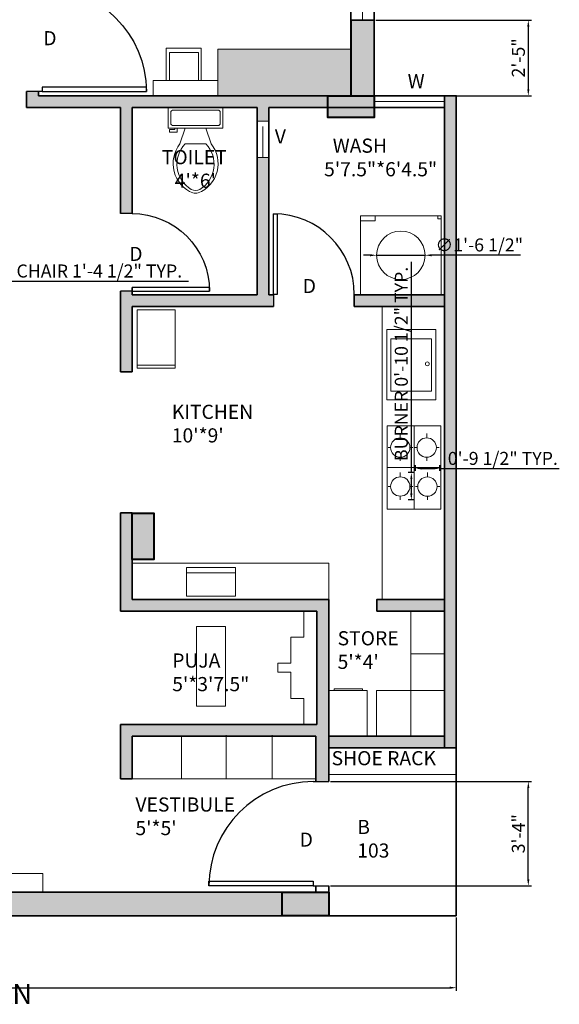
# Model space of a CAD drawing. Units: inches. Extents: x 351 to 1945, y 4338 to 4989.
# Tile 2 of 4: x 633 to 841, y 4338 to 4716. Entities that reach past the tile are written whole.
import ezdxf

# ---------------------------------------------------------------- set-up
doc = ezdxf.new("R2010")
doc.units = ezdxf.units.IN
doc.linetypes.add('ACAD_ISO02W100', pattern=[15, 12, -3])
for name, color, linetype, lineweight in [('A-ANNO-DIMS', 55, 'Continuous', 18), ('A-ANNO-IDEN', 55, 'Continuous', 18), ('A-ANNO-TEXT', 55, 'Continuous', 25), ('A-AREA-IDEN', 55, 'Continuous', 18), ('A-COLS-PATT', 210, 'Continuous', 13), ('A-EQPM', 8, 'Continuous', 18), ('A-FLOR-CASE', 30, 'Continuous', 20), ('A-FLOR-CASE-PATT', 30, 'Continuous', 13), ('A-FLOR-FIXT', 9, 'Continuous', 18), ('A-GLAZ-HIDN', 10, 'ACAD_ISO02W100', 18), ('A-WALL-PATT', 130, 'Continuous', 13), ('COLUMN', 210, 'Continuous', 40), ('DOOR', 52, 'Continuous', 25), ('FUR', 142, 'Continuous', 18), ('WALL', 130, 'Continuous', 35), ('WIND', 10, 'Continuous', 20)]:
    doc.layers.add(name, color=color, linetype=linetype, lineweight=lineweight)
doc.styles.get("Standard").update_dxf_attribs({"font": 'arial.ttf'})
doc.dimstyles.new('ISO-25', dxfattribs={"dimtxt": 5, "dimasz": 2.5, "dimexe": 1.25, "dimexo": 0.625, "dimtad": 1, "dimdec": 0, "dimlunit": 4, "dimtxsty": 'Standard', "dimcen": 2.5, "dimadec": 0, "dimazin": 0, "dimtfac": 1, "dimtdec": 0, "dimtmove": 0, "dimatfit": 3, "dimfxl": 1, "dimarcsym": 0})

# ---------------------------------------------------------------- blocks, each defined once
blk = doc.blocks.new('*U2')
for p, q in [((0, 0), (0, -6)), ((40, 0), (40, -6))]:
    blk.add_line(p, q)
blk.add_lwpolyline([(0, 0), (0, 40), (1.75, 40), (1.75, 0)], close=True)
blk.add_arc((0, 0), 40, 0, 90)
blk = doc.blocks.new('*U4')
for p, q in [((9.5, -6), (9.5, -2)), ((-10, -8.5), (-8, -8.5)), ((-10, -9.5), (-10, -8.5)), ((-7, -9.5), (-10, -9.5)), ((-8, -8.5), (-8, -8)), ((-7, -8), (-7, -9.5)), ((-4, -8), (-6, -14)), ((4, -8), (6, -14)), ((4, -14), (-4, -14))]:
    blk.add_line(p, q)
blk.add_lwpolyline([(10.5, -8), (10.5, 0), (-10.5, 0), (-10.5, -8)], close=True)
for points in [[(-9.5, -2), (-9.5, -6)], [(8.5, -1), (-8.5, -1)], [(-8.5, -7), (8.5, -7)]]:
    blk.add_lwpolyline(points)
for centre, radius, start, end in [((-8.62, -1.88), 0.884, 81.8699, 188.1301), ((8.62, -1.88), 0.884, 351.8699, 98.1301), ((-8.62, -6.12), 0.884, 171.8699, 278.1301), ((8.62, -6.12), 0.884, 261.8699, 8.1301), ((3.52, -21.58), 12.17, 141.4691, 247.9714), ((4.2, -21.82), 11.33, 136.3677, 238.9468), ((-3.52, -21.58), 12.17, 292.0284, 38.5307), ((-4.2, -21.82), 11.33, 301.053, 43.6321), ((0, -27.88), 4, 245.7318, 294.2682), ((0, -29), 4, 254.8605, 285.1395)]:
    blk.add_arc(centre, radius, start, end)
blk = doc.blocks.new('BEDROOM-DESK-AND-SEAT')
for p, q in [((5, 5.84), (5, 18.2)), ((5, 18.2), (18.5, 18.2)), ((18.5, 18.2), (18.5, 5.84))]:
    blk.add_line(p, q)
for points in [[(6.28, 5.84), (17.4, 5.84), (17.4, 16.62), (6.28, 16.62)], [(0, 0), (24.89, 0), (24.89, 5.84), (0, 5.84)]]:
    blk.add_lwpolyline(points, close=True)
blk = doc.blocks.new('WIN-49')
blk.add_line((0, 4.5), (49.03, 4.5))
blk.add_lwpolyline([(0, 0), (49.03, 0), (49.03, 9), (0, 9)], close=True)
blk = doc.blocks.new('COOKTOP-BURNER')
for p, q in [((4.6, 8.82), (4.6, 10.51)), ((0.89, 5.11), (0, 5.11)), ((8.32, 5.11), (9.37, 5.11)), ((4.6, 1.39), (4.6, 0))]:
    blk.add_line(p, q)
blk.add_circle((4.6, 5.11), 3.72)
blk = doc.blocks.new('*D15')
at = {"layer": 'A-ANNO-DIMS', "color": 0, "lineweight": -2, "transparency": 16777216}
for p, q in [((586.22, 4617.77), (586.22, 4614.71)), ((588.72, 4615.96), (599.99, 4615.96)), ((602.49, 4617.77), (602.49, 4614.71)), ((602.49, 4615.96), (698.18, 4615.96))]:
    blk.add_line(p, q, dxfattribs=at)
at = {"layer": 'A-ANNO-DIMS', "color": 0, "lineweight": 100, "transparency": 16777216}
for points in [[(588.72, 4616.38), (588.72, 4615.54), (586.22, 4615.96)], [(599.99, 4616.38), (599.99, 4615.54), (602.49, 4615.96)]]:
    blk.add_solid(points, dxfattribs=at)
at = {"layer": 'Defpoints', "color": 0, "lineweight": 100, "transparency": 16777216}
for p in [(586.22, 4618.4), (602.49, 4618.4), (602.49, 4615.96)]:
    blk.add_point(p, dxfattribs=at)
at = {"layer": 'A-ANNO-DIMS', "color": 0, "transparency": 16777216, "insert": (651.59, 4619.17), "char_height": 5, "attachment_point": 5}
blk.add_mtext('DINING CHAIR 1\'-4 1/2" TYP.', dxfattribs=at)
blk = doc.blocks.new('*D19')
at = {"layer": 'A-ANNO-DIMS', "color": 0, "lineweight": -2, "transparency": 16777216}
for p, q in [((783.81, 4542.4), (783.81, 4623.38)), ((784.76, 4542.4), (782.56, 4542.4)), ((783.81, 4534.39), (783.81, 4539.9)), ((784.76, 4531.89), (782.56, 4531.89))]:
    blk.add_line(p, q, dxfattribs=at)
at = {"layer": 'A-ANNO-DIMS', "color": 0, "lineweight": 100, "transparency": 16777216}
for points in [[(783.39, 4539.9), (784.22, 4539.9), (783.81, 4542.4)], [(783.39, 4534.39), (784.22, 4534.39), (783.81, 4531.89)]]:
    blk.add_solid(points, dxfattribs=at)
at = {"layer": 'Defpoints', "color": 0, "lineweight": 100, "transparency": 16777216}
for p in [(783.81, 4542.4), (785.38, 4542.4), (785.38, 4531.89)]:
    blk.add_point(p, dxfattribs=at)
at = {"layer": 'A-ANNO-DIMS', "color": 0, "transparency": 16777216, "insert": (780.6, 4584.14), "char_height": 5, "attachment_point": 5, "rotation": 90}
blk.add_mtext('BURNER 0\'-10 1/2" TYP.', dxfattribs=at)
blk = doc.blocks.new('*D20')
at = {"layer": 'A-ANNO-DIMS', "color": 0, "lineweight": -2, "transparency": 16777216}
for p, q in [((785.38, 4543.02), (785.38, 4545.23)), ((787.88, 4543.98), (792.26, 4543.98)), ((794.76, 4543.02), (794.76, 4545.23)), ((794.76, 4543.98), (840.64, 4543.98))]:
    blk.add_line(p, q, dxfattribs=at)
at = {"layer": 'A-ANNO-DIMS', "color": 0, "lineweight": 100, "transparency": 16777216}
for points in [[(787.88, 4544.39), (787.88, 4543.56), (785.38, 4543.98)], [(792.26, 4544.39), (792.26, 4543.56), (794.76, 4543.98)]]:
    blk.add_solid(points, dxfattribs=at)
at = {"layer": 'Defpoints', "color": 0, "lineweight": 100, "transparency": 16777216}
for p in [(794.76, 4543.98), (785.38, 4542.4), (794.76, 4542.4)]:
    blk.add_point(p, dxfattribs=at)
at = {"layer": 'A-ANNO-DIMS', "color": 0, "transparency": 16777216, "insert": (818.95, 4547.19), "char_height": 5, "attachment_point": 5}
blk.add_mtext('0\'-9 1/2" TYP.', dxfattribs=at)
blk = doc.blocks.new('*D31')
at = {"layer": 'A-ANNO-DIMS', "color": 0, "lineweight": -2, "transparency": 16777216}
for p, q in [((402.08, 4469.03), (402.08, 4343.26)), ((801.08, 4371.53), (801.08, 4343.26)), ((404.58, 4344.51), (798.58, 4344.51))]:
    blk.add_line(p, q, dxfattribs=at)
at = {"layer": 'A-ANNO-DIMS', "color": 0, "lineweight": 100, "transparency": 16777216}
for points in [[(404.58, 4344.93), (404.58, 4344.09), (402.08, 4344.51)], [(798.58, 4344.93), (798.58, 4344.09), (801.08, 4344.51)]]:
    blk.add_solid(points, dxfattribs=at)
at = {"layer": 'Defpoints', "color": 0, "lineweight": 100, "transparency": 16777216}
for p in [(402.08, 4469.66), (801.08, 4372.16), (801.08, 4344.51)]:
    blk.add_point(p, dxfattribs=at)
at = {"layer": 'A-ANNO-DIMS', "color": 0, "transparency": 16777216, "insert": (601.58, 4347.69), "char_height": 5, "attachment_point": 5}
blk.add_mtext('33\'-3"', dxfattribs=at)
blk = doc.blocks.new('*D32')
at = {"layer": 'A-ANNO-DIMS', "color": 0, "lineweight": -2, "transparency": 16777216}
for p, q in [((770.21, 4716.2), (829.98, 4716.2)), ((828.73, 4713.7), (828.73, 4689.66)), ((770.21, 4687.16), (829.98, 4687.16))]:
    blk.add_line(p, q, dxfattribs=at)
at = {"layer": 'A-ANNO-DIMS', "color": 0, "lineweight": 100, "transparency": 16777216}
for points in [[(828.32, 4713.7), (829.15, 4713.7), (828.73, 4716.2)], [(828.32, 4689.66), (829.15, 4689.66), (828.73, 4687.16)]]:
    blk.add_solid(points, dxfattribs=at)
at = {"layer": 'Defpoints', "color": 0, "lineweight": 100, "transparency": 16777216}
for p in [(769.58, 4716.2), (769.58, 4687.16), (828.73, 4687.16)]:
    blk.add_point(p, dxfattribs=at)
at = {"layer": 'A-ANNO-DIMS', "color": 0, "transparency": 16777216, "insert": (825.56, 4701.68), "char_height": 5, "attachment_point": 5, "rotation": 90}
blk.add_mtext('2\'-5"', dxfattribs=at)
blk = doc.blocks.new('*D38')
at = {"layer": 'A-ANNO-DIMS', "color": 0, "lineweight": -2, "transparency": 16777216}
for p, q in [((752.71, 4423.66), (829.98, 4423.66)), ((828.73, 4386.16), (828.73, 4421.16)), ((752.71, 4383.66), (829.98, 4383.66))]:
    blk.add_line(p, q, dxfattribs=at)
at = {"layer": 'A-ANNO-DIMS', "color": 0, "lineweight": 100, "transparency": 16777216}
for points in [[(828.32, 4421.16), (829.15, 4421.16), (828.73, 4423.66)], [(828.32, 4386.16), (829.15, 4386.16), (828.73, 4383.66)]]:
    blk.add_solid(points, dxfattribs=at)
at = {"layer": 'Defpoints', "color": 0, "lineweight": 100, "transparency": 16777216}
for p in [(752.08, 4423.66), (828.73, 4423.66), (752.08, 4383.66)]:
    blk.add_point(p, dxfattribs=at)
at = {"layer": 'A-ANNO-DIMS', "color": 0, "transparency": 16777216, "insert": (825.56, 4403.66), "char_height": 5, "attachment_point": 5, "rotation": 90}
blk.add_mtext('3\'-4"', dxfattribs=at)
blk = doc.blocks.new('*D52')
at = {"layer": 'A-ANNO-DIMS', "color": 0, "lineweight": -2, "transparency": 16777216}
for p, q in [((767.96, 4625.86), (765.46, 4625.86)), ((770.46, 4625.86), (789.1, 4625.86)), ((825.73, 4625.86), (791.6, 4625.86))]:
    blk.add_line(p, q, dxfattribs=at)
at = {"layer": 'A-ANNO-DIMS', "color": 0, "lineweight": 100, "transparency": 16777216}
for points in [[(767.96, 4626.28), (767.96, 4625.45), (770.46, 4625.86)], [(791.6, 4626.28), (791.6, 4625.45), (789.1, 4625.86)]]:
    blk.add_solid(points, dxfattribs=at)
at = {"layer": 'Defpoints', "color": 0, "lineweight": 100, "transparency": 16777216}
for p in [(770.46, 4625.86), (789.1, 4625.86)]:
    blk.add_point(p, dxfattribs=at)
at = {"layer": 'A-ANNO-DIMS', "color": 0, "transparency": 16777216, "insert": (809.91, 4629.18), "char_height": 5, "attachment_point": 5, "rotation": 0.0029}
blk.add_mtext('∅1\'-6 1/2"', dxfattribs=at)

msp = doc.modelspace()

# ---------------------------------------------------------------- hatches: boundary and pattern name
at = {"layer": 'A-COLS-PATT'}
h = msp.add_hatch(color=256, dxfattribs=at)
h.dxf.hatch_style = 1
h.paths.add_polyline_path([(419.45, 4819.16), (411.08, 4819.16), (411.08, 4801.31), (419.45, 4801.31)])
h.paths.add_polyline_path([(760.58, 4819.16), (752.22, 4819.16), (752.22, 4801.31), (760.58, 4801.31)])
h.paths.add_polyline_path([(567.08, 4819.16), (558.72, 4819.16), (558.72, 4801.31), (567.08, 4801.31)])
h.paths.add_polyline_path([(423.85, 4675.88), (411.08, 4675.88), (411.08, 4669.65), (423.85, 4669.65)])
h.paths.add_polyline_path([(575.47, 4670.66), (567.1, 4670.66), (567.1, 4658.77), (575.47, 4658.77)])
h.paths.add_polyline_path([(575.47, 4676.62), (570.08, 4676.62), (567.1, 4676.62), (567.1, 4670.66), (575.47, 4670.66)])
h.paths.add_polyline_path([(769.58, 4687.16), (751.73, 4687.16), (751.73, 4682.66), (769.58, 4682.66)])
h.paths.add_polyline_path([(769.58, 4682.66), (751.73, 4682.66), (751.73, 4678.79), (769.58, 4678.79)])
h.paths.add_polyline_path([(514.67, 4381.16), (502.58, 4381.16), (502.58, 4372.16), (514.67, 4372.16)])
h.paths.add_polyline_path([(624.15, 4381.16), (606.3, 4381.16), (606.3, 4372.16), (624.15, 4372.16)])
h.paths.add_polyline_path([(752.08, 4381.16), (734.23, 4381.16), (734.23, 4372.16), (752.08, 4372.16)])
h.paths.add_polyline_path([(684.94, 4526.8), (676.58, 4526.8), (676.58, 4508.95), (684.94, 4508.95)])
h.paths.add_polyline_path([(419.45, 4492.01), (411.08, 4492.01), (411.08, 4474.16), (419.45, 4474.16)])
h.paths.add_polyline_path([(414.54, 4480.61), (443.82, 4480.61), (443.82, 4500.88), (414.54, 4500.88)], flags=9)
at = {"layer": 'A-FLOR-CASE-PATT'}
h = msp.add_hatch(color=256, dxfattribs=at)
h.dxf.hatch_style = 1
h.paths.add_polyline_path([(440.18, 4819.16), (419.45, 4819.16), (419.45, 4801.31), (411.08, 4801.31), (411.08, 4729.12), (440.18, 4729.12)])
h.paths.add_polyline_path([(760.58, 4704.97), (709.51, 4704.97), (709.51, 4687.16), (760.58, 4687.16)])
h.paths.add_polyline_path([(555.08, 4624.13), (533.62, 4624.13), (533.62, 4538.66), (546.72, 4538.66), (546.72, 4556.51), (555.08, 4556.51)])
at = {"layer": 'A-WALL-PATT'}
h = msp.add_hatch(color=256, dxfattribs=at)
h.dxf.hatch_style = 1
h.paths.add_polyline_path([(519.58, 4828.16), (519.58, 4819.16), (534.65, 4819.16), (567.08, 4819.16), (567.08, 4801.31), (567.08, 4783.74), (571.99, 4783.74), (576.08, 4783.74), (576.08, 4819.16), (636.08, 4819.16), (636.08, 4728.72), (640.58, 4728.72), (640.58, 4819.16), (684.63, 4819.16), (684.63, 4828.16), (640.58, 4828.16), (576.08, 4828.16)])
h.paths.add_polyline_path([(402.08, 4828.16), (402.08, 4749.41), (411.08, 4749.41), (411.08, 4819.16), (419.45, 4819.16), (470.55, 4819.16), (470.55, 4828.16)])
h.paths.add_polyline_path([(733.65, 4828.16), (733.65, 4819.16), (746.53, 4819.16), (760.58, 4819.16), (760.58, 4801.31), (760.58, 4765.23), (769.58, 4765.23), (769.58, 4828.16)])
h.paths.add_polyline_path([(402.08, 4670.66), (402.08, 4623.83), (411.08, 4623.83), (411.08, 4670.66), (411.08, 4675.88), (411.08, 4700.38), (402.08, 4700.38)])
h.paths.add_polyline_path([(555.08, 4670.66), (555.08, 4667.68), (559.58, 4667.68), (559.58, 4670.66), (567.1, 4670.66), (567.1, 4675.16), (423.95, 4675.16), (423.85, 4675.16), (423.85, 4670.66)])
h.paths.add_polyline_path([(576.08, 4727.66), (576.08, 4751.3, -0.031413), (571.99, 4751.04), (567.08, 4751.04), (567.08, 4716.51, -0.01877), (570.08, 4716.62), (576.08, 4716.62), (576.08, 4723.16), (636.08, 4723.16), (640.58, 4723.16), (640.58, 4728.72), (636.08, 4728.72), (636.08, 4727.66)])
h.paths.add_polyline_path([(672.08, 4682.66), (672.08, 4641.87), (676.58, 4641.87), (676.58, 4682.66), (724.58, 4682.66), (724.58, 4677.41), (729.08, 4677.41), (729.08, 4682.66), (751.73, 4682.66), (751.73, 4687.16), (709.51, 4687.16), (684.61, 4687.16), (640.58, 4687.16), (640.58, 4688.72), (636.08, 4688.72), (636.08, 4682.66)])
h.paths.add_polyline_path([(753.8, 4463.91), (782.66, 4463.91), (782.66, 4484.16), (753.8, 4484.16)], flags=9)
h.paths.add_polyline_path([(760.86, 4391.5), (776.24, 4391.5), (776.24, 4411.77), (760.86, 4411.77)], flags=9)
h.paths.add_polyline_path([(690.04, 4455.43), (720.56, 4455.43), (720.56, 4475.7), (690.04, 4475.7)], flags=9)
h.paths.add_polyline_path([(676.19, 4400.06), (720.94, 4400.06), (720.94, 4420.3), (676.19, 4420.3)], flags=9)
h.paths.add_polyline_path([(550.38, 4425.45), (615.73, 4425.45), (615.73, 4445.72), (550.38, 4445.72)], flags=9)
h.paths.add_polyline_path([(417.92, 4480.61), (447.2, 4480.61), (447.2, 4500.88), (417.92, 4500.88)], flags=9)
h.paths.add_polyline_path([(449.69, 4582.66), (497.94, 4582.66), (497.94, 4602.93), (449.69, 4602.93)], flags=9)
h.paths.add_polyline_path([(580.8, 4638.02), (622.18, 4638.02), (622.18, 4658.29), (580.8, 4658.29)], flags=9)
h.paths.add_polyline_path([(748.64, 4653.12), (792.13, 4653.12), (792.13, 4673.39), (748.64, 4673.39)], flags=9)
h.paths.add_polyline_path([(686.44, 4648.7), (715.72, 4648.7), (715.72, 4668.97), (686.44, 4668.97)], flags=25)
h.paths.add_polyline_path([(689.64, 4550.87), (725.93, 4550.87), (725.93, 4571.14), (689.64, 4571.14)], flags=9)
h.paths.add_polyline_path([(671.27, 4732.55), (719.52, 4732.55), (719.52, 4752.82), (671.27, 4752.82)], flags=9)
h.paths.add_polyline_path([(458.57, 4731.55), (540.55, 4731.55), (540.55, 4751.82), (458.57, 4751.82)], flags=9)
h = msp.add_hatch(color=256, dxfattribs=at)
h.dxf.hatch_style = 1
h.paths.add_polyline_path([(729.08, 4663.38), (724.58, 4663.38), (724.58, 4610.66), (676.58, 4610.66), (676.58, 4612.12), (676.55, 4612.12), (672.08, 4612.12), (672.08, 4606.16), (672.08, 4581.14), (676.58, 4581.14), (676.58, 4606.16), (729.08, 4606.16), (730.91, 4606.16), (730.91, 4610.66), (729.08, 4610.66)])
h.paths.add_polyline_path([(676.58, 4507.65), (676.58, 4508.95), (676.58, 4508.95), (676.58, 4526.98), (672.08, 4526.98), (672.08, 4489.16), (676.58, 4489.16), (687.08, 4489.16), (747.58, 4489.16), (747.58, 4445.66), (742.58, 4445.66), (687.08, 4445.66), (676.58, 4445.66), (672.08, 4445.66), (672.08, 4424.71), (676.58, 4424.71), (676.58, 4441.16), (687.08, 4441.16), (747.08, 4441.16), (747.08, 4423.66), (752.08, 4423.66), (752.08, 4445.66), (752.08, 4458.62), (752.08, 4489.16), (752.08, 4493.66), (676.58, 4493.66)])
h.paths.add_polyline_path([(734.23, 4381.16), (687.08, 4381.16), (680.85, 4381.16), (624.15, 4381.16), (624.15, 4372.16), (687.08, 4372.16), (734.23, 4372.16)])
h.paths.add_polyline_path([(606.3, 4381.16), (570.36, 4381.16), (563.7, 4381.16), (563.7, 4372.16), (606.3, 4372.16)])
h.paths.add_polyline_path([(753.8, 4463.91), (782.66, 4463.91), (782.66, 4484.16), (753.8, 4484.16)], flags=9)
h.paths.add_polyline_path([(760.86, 4391.5), (776.24, 4391.5), (776.24, 4411.77), (760.86, 4411.77)], flags=9)
h.paths.add_polyline_path([(690.04, 4455.43), (720.56, 4455.43), (720.56, 4475.7), (690.04, 4475.7)], flags=25)
h.paths.add_polyline_path([(676.19, 4400.06), (720.94, 4400.06), (720.94, 4420.3), (676.19, 4420.3)], flags=9)
h.paths.add_polyline_path([(550.38, 4425.45), (615.73, 4425.45), (615.73, 4445.72), (550.38, 4445.72)], flags=9)
h.paths.add_polyline_path([(417.92, 4480.61), (447.2, 4480.61), (447.2, 4500.88), (417.92, 4500.88)], flags=9)
h.paths.add_polyline_path([(449.69, 4582.66), (497.94, 4582.66), (497.94, 4602.93), (449.69, 4602.93)], flags=9)
h.paths.add_polyline_path([(580.8, 4638.02), (622.18, 4638.02), (622.18, 4658.29), (580.8, 4658.29)], flags=9)
h.paths.add_polyline_path([(748.64, 4653.12), (792.13, 4653.12), (792.13, 4673.39), (748.64, 4673.39)], flags=9)
h.paths.add_polyline_path([(686.44, 4648.7), (715.72, 4648.7), (715.72, 4668.97), (686.44, 4668.97)], flags=9)
h.paths.add_polyline_path([(689.64, 4550.87), (725.93, 4550.87), (725.93, 4571.14), (689.64, 4571.14)], flags=9)
h.paths.add_polyline_path([(671.27, 4732.55), (719.52, 4732.55), (719.52, 4752.82), (671.27, 4752.82)], flags=9)
h.paths.add_polyline_path([(594.05, 4791.87), (624.3, 4791.87), (624.3, 4812.11), (594.05, 4812.11)], flags=9)
h.paths.add_polyline_path([(458.57, 4731.55), (540.55, 4731.55), (540.55, 4751.82), (458.57, 4751.82)], flags=9)
h = msp.add_hatch(color=256, dxfattribs=at)
h.dxf.hatch_style = 1
h.paths.add_polyline_path([(769.58, 4716.2), (760.66, 4716.2), (760.66, 4687.16), (769.58, 4687.16)])
h.paths.add_polyline_path([(801.08, 4687.16), (796.58, 4687.16), (796.58, 4436.66), (801.08, 4436.66)])
h.paths.add_polyline_path([(411.08, 4574.8), (402.08, 4574.8), (402.08, 4534.16), (411.08, 4534.16), (411.08, 4538.66)])
h.paths.add_polyline_path([(411.08, 4534.16), (402.08, 4534.16), (402.08, 4517.84), (411.08, 4517.84)])
h.paths.add_polyline_path([(435.45, 4538.66), (411.08, 4538.66), (411.08, 4534.16), (435.45, 4534.16)])
h.paths.add_polyline_path([(411.08, 4492.45), (402.08, 4492.45), (402.08, 4469.66), (411.08, 4469.66)])
h.paths.add_polyline_path([(498.08, 4474.16), (411.08, 4474.16), (411.08, 4469.66), (498.08, 4469.66)])
h.paths.add_polyline_path([(502.58, 4534.16), (498.08, 4534.16), (498.08, 4466.28), (502.58, 4466.28)])
h.paths.add_polyline_path([(533.62, 4538.66), (465.58, 4538.66), (465.58, 4534.16), (533.62, 4534.16)])
h.paths.add_polyline_path([(559.58, 4627.68), (555.08, 4627.68), (555.08, 4538.66), (546.72, 4538.66), (533.62, 4538.66), (533.62, 4534.16), (559.58, 4534.16)])
h = msp.add_hatch(color=256, dxfattribs=at)
h.dxf.hatch_style = 1
h.paths.add_polyline_path([(796.58, 4610.66), (761.9, 4610.66), (761.9, 4606.16), (796.58, 4606.16)])
h = msp.add_hatch(color=256, dxfattribs=at)
h.dxf.hatch_style = 1
h.paths.add_polyline_path([(796.58, 4493.66), (770.57, 4493.66), (770.57, 4489.16), (796.58, 4489.16)])
h.paths.add_polyline_path([(796.58, 4441.16), (752.08, 4441.16), (752.08, 4436.66), (796.58, 4436.66)])

# ---------------------------------------------------------------- linework, layer by layer
at = {"layer": 'A-EQPM'}
for p, q in [((784.87, 4528.27), (784.87, 4560.33)), ((774.58, 4544.3), (795.16, 4544.3)), ((697.47, 4503.9), (716.34, 4503.9))]:
    msp.add_line(p, q, dxfattribs=at)
for points in [[(764.34, 4610.66), (795.22, 4610.66), (795.22, 4641.07), (764.34, 4641.07)], [(764.34, 4639.13), (769.94, 4639.13), (769.94, 4641.07), (764.34, 4641.07)], [(795.22, 4641.07), (793.98, 4641.07), (793.98, 4639.88), (795.22, 4639.88)], [(795.22, 4641.07), (795.22, 4641.07), (795.22, 4639.44), (795.22, 4639.44)], [(678.55, 4583.6), (693.06, 4583.6), (693.06, 4604.89), (678.55, 4604.89)], [(678.55, 4583.6), (693.06, 4583.6), (693.06, 4582.45), (678.55, 4582.45)], [(774.58, 4560.33), (795.16, 4560.33), (795.16, 4528.27), (774.58, 4528.27)], [(697.47, 4505.87), (716.34, 4505.87), (716.34, 4494.91), (697.47, 4494.91)]]:
    msp.add_lwpolyline(points, close=True, dxfattribs=at)
msp.add_circle((779.78, 4625.86), 9.32, dxfattribs=at)
at = {"layer": 'A-FLOR-CASE'}
for p, q in [((796.58, 4606.16), (772.58, 4606.16)), ((772.58, 4606.16), (772.58, 4493.66)), ((745.58, 4489.16), (742.58, 4489.16)), ((742.58, 4489.16), (742.58, 4484.16)), ((742.58, 4489.16), (742.58, 4484.16)), ((747.58, 4489.16), (745.58, 4489.16)), ((783.58, 4489.16), (783.58, 4441.16)), ((742.58, 4484.16), (742.58, 4479.16)), ((742.58, 4479.16), (737.58, 4479.16)), ((737.58, 4479.16), (737.58, 4469.16)), ((783.58, 4472.71), (796.58, 4472.71)), ((737.58, 4469.16), (732.58, 4469.16)), ((732.58, 4469.16), (732.58, 4465.66)), ((732.58, 4465.66), (737.58, 4465.66)), ((737.58, 4460.66), (737.58, 4465.66)), ((737.58, 4455.66), (737.58, 4460.66)), ((742.58, 4455.66), (737.58, 4455.66)), ((742.58, 4450.66), (742.58, 4455.66)), ((766.85, 4458.62), (752.08, 4458.62)), ((796.58, 4458.62), (770.46, 4458.62)), ((770.46, 4458.62), (770.46, 4441.16)), ((742.58, 4445.66), (742.58, 4450.66)), ((747.58, 4445.66), (742.58, 4445.66)), ((695.56, 4424.71), (695.56, 4441.16)), ((712.76, 4425.01), (712.76, 4441.46)), ((730.34, 4425.01), (730.34, 4441.46)), ((752.08, 4426.35), (801.08, 4426.35)), ((747.08, 4424.71), (676.58, 4424.71))]:
    msp.add_line(p, q, dxfattribs=at)
for points in [[(709.51, 4687.16), (760.58, 4687.16), (760.58, 4704.97), (709.51, 4704.97)], [(752.08, 4493.66), (676.58, 4493.66), (676.58, 4507.65), (752.08, 4507.65)], [(712.44, 4452.65), (701.29, 4452.65), (701.29, 4483.24), (712.44, 4483.24)], [(754.17, 4458.62), (765.07, 4458.62), (765.07, 4459.35), (754.17, 4459.35)], [(752.08, 4441.16), (766.85, 4441.16), (766.85, 4458.62), (752.08, 4458.62)], [(570.36, 4381.16), (642.24, 4381.16), (642.24, 4388.42), (570.36, 4388.42)]]:
    msp.add_lwpolyline(points, close=True, dxfattribs=at)
at = {"layer": 'A-FLOR-FIXT'}
for points in [[(793.28, 4597.29), (774.37, 4597.29), (774.37, 4570.36), (793.28, 4570.36)], [(775.94, 4573.6), (791.61, 4573.6), (791.61, 4593.75), (775.94, 4593.75)]]:
    msp.add_lwpolyline(points, close=True, dxfattribs=at)
msp.add_circle((789.94, 4584.15), 0.75, dxfattribs=at)
at = {"layer": 'A-GLAZ-HIDN'}
msp.add_line((726.83, 4663.38), (726.83, 4677.41), dxfattribs=at)
msp.add_lwpolyline([(724.58, 4677.41), (729.08, 4677.41), (729.08, 4663.38), (724.58, 4663.38)], close=True, dxfattribs=at)
at = {"layer": 'COLUMN'}
for points in [[(769.58, 4687.16), (769.58, 4678.79), (751.73, 4678.79), (751.73, 4687.16)], [(676.58, 4526.8), (684.94, 4526.8), (684.94, 4508.95), (676.58, 4508.95)], [(752.08, 4381.16), (752.08, 4372.16), (734.23, 4372.16), (734.23, 4381.16)]]:
    msp.add_lwpolyline(points, close=True, dxfattribs=at)
at = {"layer": 'WALL'}
for p, q in [((769.58, 4828.16), (769.58, 4687.16)), ((760.58, 4819.16), (760.58, 4687.16)), ((636.08, 4682.66), (636.08, 4688.72)), ((640.58, 4687.16), (640.58, 4688.72)), ((760.58, 4687.16), (640.58, 4687.16)), ((769.58, 4687.16), (801.08, 4687.16)), ((801.08, 4687.16), (801.08, 4606.16)), ((672.08, 4682.66), (636.08, 4682.66)), ((672.08, 4682.66), (672.08, 4641.87)), ((676.58, 4682.66), (676.58, 4641.87)), ((724.58, 4682.66), (676.58, 4682.66)), ((724.58, 4610.66), (724.58, 4682.66)), ((769.58, 4682.66), (729.08, 4682.66)), ((729.08, 4610.66), (729.08, 4682.66)), ((729.08, 4682.66), (796.58, 4682.66)), ((729.08, 4682.66), (796.58, 4682.66)), ((796.58, 4682.66), (796.58, 4610.66)), ((796.58, 4682.66), (796.58, 4610.66)), ((676.58, 4670.66), (676.58, 4646.84)), ((672.08, 4612.12), (672.08, 4606.16)), ((676.58, 4613.42), (676.58, 4610.66)), ((676.58, 4610.66), (724.58, 4610.66)), ((729.08, 4610.66), (730.91, 4610.66)), ((761.9, 4610.66), (796.58, 4610.66)), ((672.08, 4606.16), (672.08, 4581.14)), ((676.58, 4606.16), (729.08, 4606.16)), ((676.58, 4606.16), (676.58, 4581.14)), ((729.08, 4606.16), (730.91, 4606.16)), ((761.9, 4606.16), (796.58, 4606.16)), ((796.58, 4606.16), (796.58, 4493.66)), ((801.08, 4606.16), (801.08, 4489.16)), ((672.08, 4581.14), (676.58, 4581.14)), ((672.08, 4526.98), (672.08, 4489.16)), ((672.08, 4526.98), (676.58, 4526.98)), ((676.58, 4526.98), (676.58, 4493.66)), ((687.08, 4493.66), (676.58, 4493.66)), ((687.08, 4493.66), (752.08, 4493.66)), ((752.08, 4489.16), (752.08, 4493.66)), ((770.57, 4493.66), (796.58, 4493.66)), ((770.57, 4493.66), (770.57, 4489.16)), ((676.58, 4489.16), (672.08, 4489.16)), ((687.08, 4489.16), (676.58, 4489.16)), ((687.08, 4489.16), (747.58, 4489.16)), ((747.58, 4489.16), (747.58, 4445.66)), ((752.08, 4489.16), (752.08, 4445.66)), ((770.57, 4489.16), (796.58, 4489.16)), ((796.58, 4489.16), (796.58, 4441.16)), ((801.08, 4372.16), (801.08, 4489.16)), ((676.58, 4445.66), (672.08, 4445.66)), ((672.08, 4445.66), (672.08, 4424.71)), ((687.08, 4445.66), (676.58, 4445.66)), ((747.58, 4445.66), (687.08, 4445.66)), ((752.08, 4423.66), (752.08, 4445.66)), ((687.08, 4441.16), (676.58, 4441.16)), ((676.58, 4441.16), (676.58, 4424.71)), ((747.08, 4441.16), (687.08, 4441.16)), ((747.08, 4423.66), (747.08, 4441.16)), ((796.58, 4441.16), (752.08, 4441.16)), ((801.08, 4436.66), (752.08, 4436.66)), ((676.58, 4424.71), (672.08, 4424.71)), ((747.08, 4381.16), (747.08, 4383.66)), ((752.08, 4372.16), (752.08, 4383.66)), ((502.58, 4381.16), (682.58, 4381.16)), ((680.85, 4381.16), (692.25, 4381.16)), ((687.08, 4381.16), (747.08, 4381.16)), ((502.58, 4372.16), (687.08, 4372.16)), ((687.08, 4372.16), (752.08, 4372.16)), ((752.08, 4372.16), (801.08, 4372.16))]:
    msp.add_line(p, q, dxfattribs=at)
for points in [[(760.66, 4687.16), (769.58, 4687.16), (769.58, 4716.2), (760.66, 4716.2)], [(796.58, 4436.66), (801.08, 4436.66), (801.08, 4687.16), (796.58, 4687.16)], [(761.9, 4606.16), (796.58, 4606.16), (796.58, 4610.66), (761.9, 4610.66)], [(770.57, 4489.16), (796.58, 4489.16), (796.58, 4493.66), (770.57, 4493.66)], [(752.08, 4436.66), (796.58, 4436.66), (796.58, 4441.16), (752.08, 4441.16)]]:
    msp.add_lwpolyline(points, close=True, dxfattribs=at)
at = {"layer": 'WIND'}
msp.add_line((769.58, 4684.91), (796.58, 4684.91), dxfattribs=at)
msp.add_lwpolyline([(769.58, 4687.16), (796.58, 4687.16), (796.58, 4682.66), (769.58, 4682.66)], close=True, dxfattribs=at)

# ---------------------------------------------------------------- block references
at = {"layer": 'A-EQPM'}
for p in [(774.97, 4546.88), (785.11, 4546.88), (774.97, 4531.93), (785.38, 4531.89)]:
    msp.add_blockref('COOKTOP-BURNER', p, dxfattribs=at)
at = {"layer": 'A-FLOR-FIXT'}
msp.add_blockref('*U4', (700.94, 4682.66), dxfattribs=at)
at = {"layer": 'DOOR', "xscale": -1, "rotation": 270}
msp.add_blockref('*U2', (642.08, 4688.72), dxfattribs=at)
at = {"layer": 'DOOR', "xscale": -0.7437101483955227, "yscale": 0.7437101483955227, "zscale": 0.7437101483955227, "rotation": 270}
msp.add_blockref('*U2', (676.55, 4612.12), dxfattribs=at)
at = {"layer": 'DOOR', "xscale": 0.7749679903478136, "yscale": 0.7749679903478136, "zscale": 0.7749679903478136}
msp.add_blockref('*U2', (730.91, 4610.81), dxfattribs=at)
at = {"layer": 'DOOR', "rotation": 90}
msp.add_blockref('*U2', (746.08, 4383.66), dxfattribs=at)
at = {"layer": 'FUR'}
msp.add_blockref('BEDROOM-DESK-AND-SEAT', (684.61, 4687.16), dxfattribs=at)
at = {"layer": 'WIND', "rotation": 270.0000000000007}
msp.add_blockref('WIN-49', (760.58, 4765.23), dxfattribs=at)

# ---------------------------------------------------------------- texts
at = {"layer": 'A-ANNO-IDEN', "char_height": 5.43, "attachment_point": 1}
for s, insert in [('D', (642.47, 4711.97)), ('W', (782.41, 4695.45)), ('V', (731.38, 4674.23)), ('D', (675.49, 4629.1)), ('D', (742.1, 4616.76)), ('D', (740.93, 4404.1))]:
    msp.add_mtext_dynamic_manual_height_columns(s, width=132.0225, gutter_width=27.16, heights=[0], dxfattribs=dict(at, insert=insert))
at = {"layer": 'A-ANNO-TEXT', "attachment_point": 1}
for s, width, gutter_width, insert, char_height in [('SHOE RACK', 132.0225, 27.16, (753.19, 4435.39), 5.432), ('3BHK PLAN', 489.8705, 38.61, (582.18, 4345.99), 7.723)]:
    msp.add_mtext_dynamic_manual_height_columns(s, width=width, gutter_width=gutter_width, heights=[0], dxfattribs=dict(at, insert=insert, char_height=char_height))
at = {"layer": 'A-AREA-IDEN', "attachment_point": 1}
for s, insert, char_height in [('  WASH\\P5\'7.5"*6\'4.5"', (750.31, 4670.68), 5.4321), ("TOILET\\P   4'*6'", (687.98, 4666.27), 5.432), ("KITCHEN\\P10'*9'", (691.82, 4568.44), 5.432), ("STORE\\P5'*4'", (755.5, 4481.46), 5.432), ('PUJA\\P5\'*3\'7.5"', (691.98, 4472.9), 5.432), ("VESTIBULE\\P5'*5'", (677.86, 4417.6), 5.432), ('B\\P103', (763.05, 4408.97), 5.432)]:
    msp.add_mtext_dynamic_manual_height_columns(s, width=132.0225, gutter_width=27.16, heights=[0], dxfattribs=dict(at, insert=insert, char_height=char_height))

# ---------------------------------------------------------------- dimensions: what is measured, and where the dimension line sits
at = {"layer": 'A-ANNO-DIMS'}
for base, p1, p2, picture, middle in [((828.73, 4687.16), (769.58, 4716.2), (769.58, 4687.16), '*D32', (825.56, 4701.68)), ((828.73, 4423.66), (752.08, 4383.66), (752.08, 4423.66), '*D38', (825.56, 4403.66))]:
    dim = msp.add_linear_dim(base=base, p1=p1, p2=p2, angle=90, dimstyle='ISO-25', override={"dimdec": 1, "dimlfac": 1, "dimrnd": 0, "dimzin": 1, "dimdsep": 46, "dimlunit": 4, "dimfrac": 2}, dxfattribs=at)
    dim.commit()
    dim.dimension.update_dxf_attribs({"geometry": picture, "text_midpoint": middle})
for base, p1, p2, text, picture, middle in [((602.49, 4615.96), (586.22, 4618.4), (602.49, 4618.4), 'DINING CHAIR <> TYP.', '*D15', (651.59, 4619.17)), ((794.76, 4543.98), (785.38, 4542.4), (794.76, 4542.4), '<> TYP.', '*D20', (818.95, 4547.19))]:
    dim = msp.add_linear_dim(base=base, p1=p1, p2=p2, text=text, dimstyle='ISO-25', override={"dimdec": 1, "dimlfac": 1, "dimrnd": 0, "dimzin": 1, "dimdsep": 46, "dimlunit": 4, "dimfrac": 2}, dxfattribs=at)
    dim.commit()
    dim.dimension.update_dxf_attribs({"geometry": picture, "text_midpoint": middle})
dim = msp.add_diameter_dim_2p(p1=(770.46, 4625.86), p2=(789.1, 4625.86), dimstyle='ISO-25', override={"dimdec": 1, "dimlfac": 1, "dimrnd": 0, "dimzin": 1, "dimdsep": 46, "dimlunit": 4, "dimfrac": 2}, dxfattribs=at)
dim.commit()
dim.dimension.update_dxf_attribs({"geometry": '*D52', "text_midpoint": (809.91, 4625.86), "dimtype": 163})
dim = msp.add_linear_dim(base=(783.81, 4542.4), p1=(785.38, 4531.89), p2=(785.38, 4542.4), angle=90, text='BURNER <> TYP.', dimstyle='ISO-25', override={"dimdec": 1, "dimlfac": 1, "dimrnd": 0, "dimzin": 1, "dimdsep": 46, "dimlunit": 4, "dimfrac": 2}, dxfattribs=at)
dim.commit()
dim.dimension.update_dxf_attribs({"geometry": '*D19', "text_midpoint": (780.6, 4584.14)})
dim = msp.add_linear_dim(base=(801.08, 4344.51), p1=(402.08, 4469.66), p2=(801.08, 4372.16), dimstyle='ISO-25', override={"dimdec": 1, "dimlfac": 1, "dimrnd": 0, "dimzin": 1, "dimdsep": 46, "dimlunit": 4, "dimfrac": 2}, dxfattribs=at)
dim.commit()
dim.dimension.update_dxf_attribs({"geometry": '*D31', "text_midpoint": (601.58, 4347.69)})

doc.saveas('drawing.dxf')
